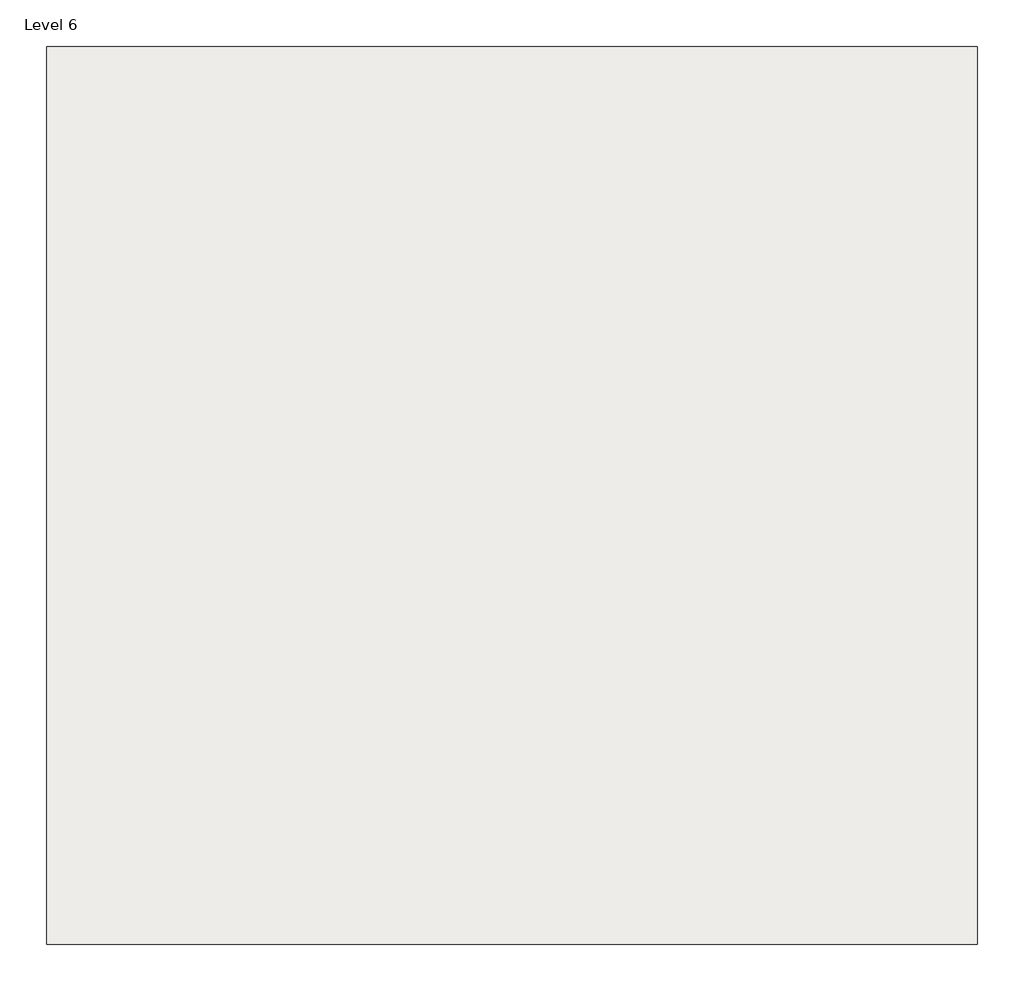
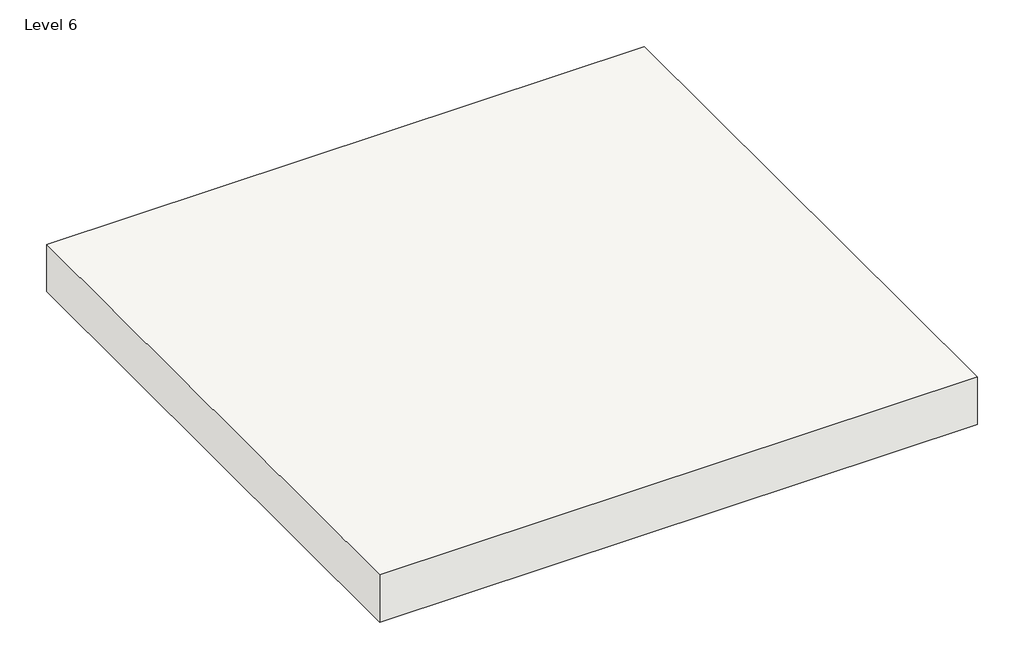
# One storey: 1 roof.
"""IFC4 building model written with IfcOpenShell, lengths in millimetres."""

from ifc_helpers import new_model, si_unit, frame, origin, place, context, project, spatial, polyline, outline, extrude, element, save

model = new_model("IFC4")

# Units and contexts
model_context = context("Model", 3, world=origin())
ifc_project = project(units=[si_unit("LENGTHUNIT", "METRE", prefix="MILLI")], contexts=[model_context])

# Site, building, storey
site = spatial("IfcSite", under=ifc_project)
building = spatial("IfcBuilding", under=site)
storey = spatial("IfcBuildingStorey", under=building, Name="Level 6", Elevation=17678.4)

# Roof
placement = place(None, origin())
element("IfcRoof", 1, ObjectType="Generic - 12\"", at=placement, inside=storey, context=model_context, shape_type="SweptSolid", body=[
    extrude(outline(polyline([(-4018.1821198, 5098.7280349), (-360.5821198, 5098.7280349), (-360.5821198, 1569.2720741), (-4018.1821198, 1569.2720741), (-4018.1821198, 5098.7280349)])), frame((0.0, 0.0, 15544.8), z_axis=(0.0, 0.0, 1.0), x_axis=(1.0, 0.0, 0.0)), (0.0, 0.0, 1.0), 304.8),
])

save(model, "model.ifc")

# Revit data of these elements
# Type "Generic - 12\""
#   Assembly Code = "B1020"
#   Layers, outside or top first: 1' - 0" no material (function 1)
# Element 1 (IfcRoof, "Generic - 12\"")
#   built-in parameter 1001705 = 52 (stored number, unit not read)
#   built-in parameter 1001701 = -7 (stored number, unit not read)
#   built-in parameter 1001710 = 33615
#   Phase Created = New Construction
#   Materials on its faces: "Default Roof"
# Materials
#   "Default Roof": colour RGB 88 101 114, transparency 0
